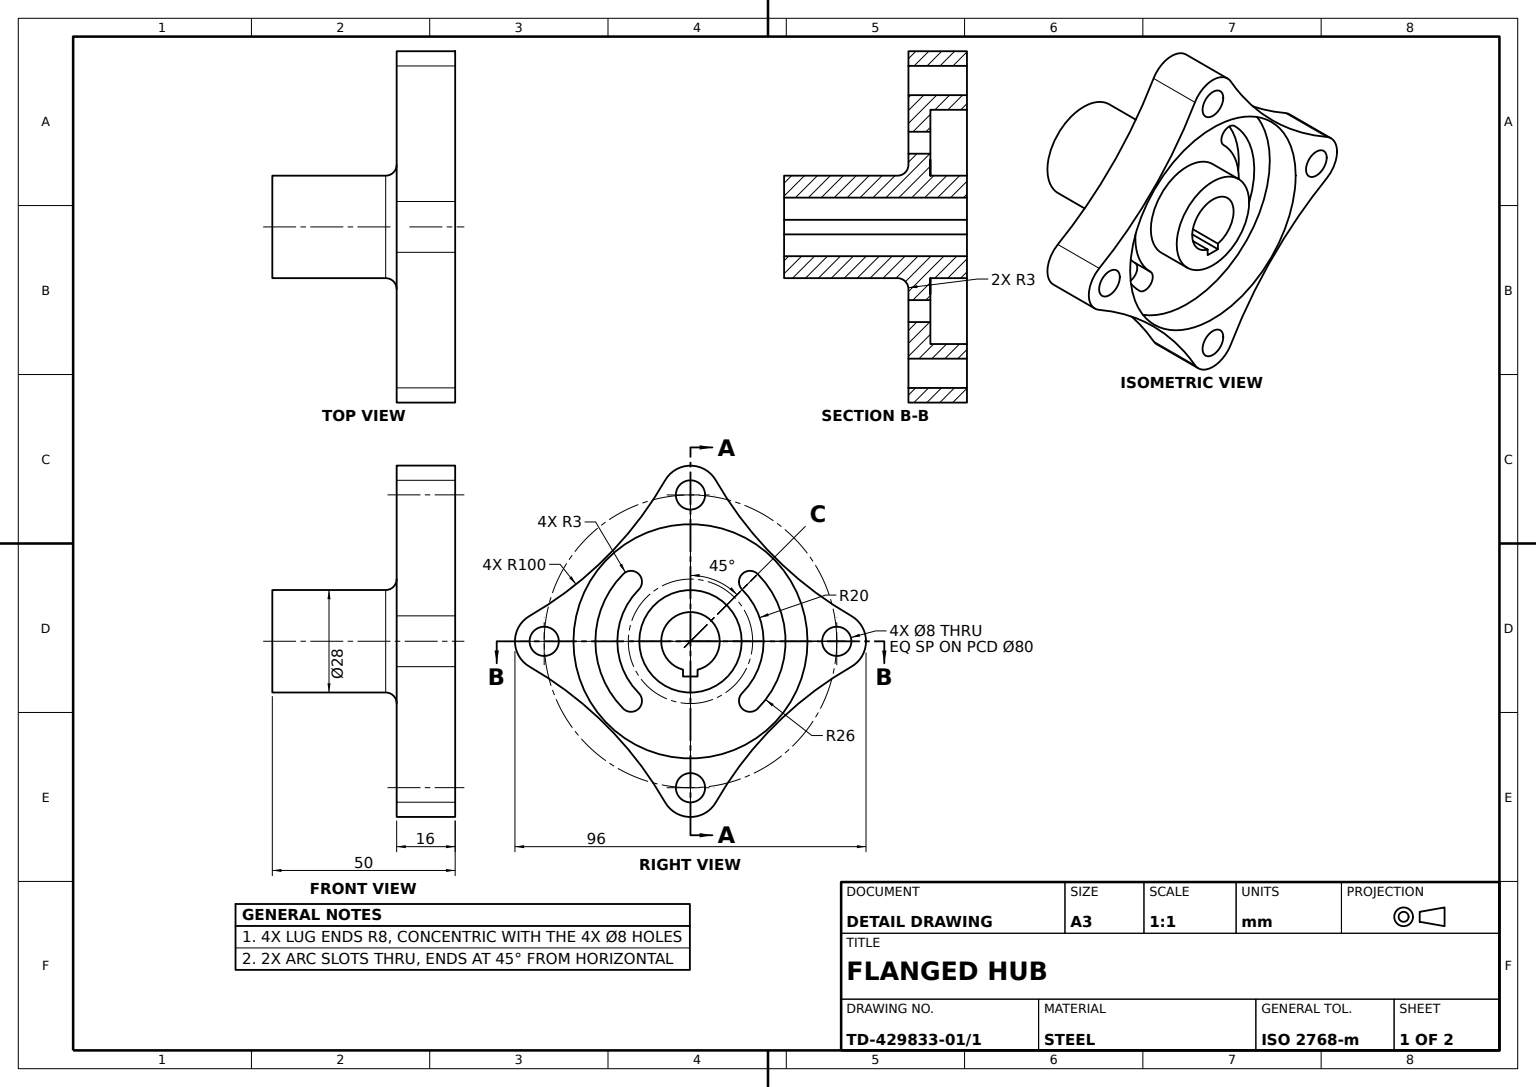
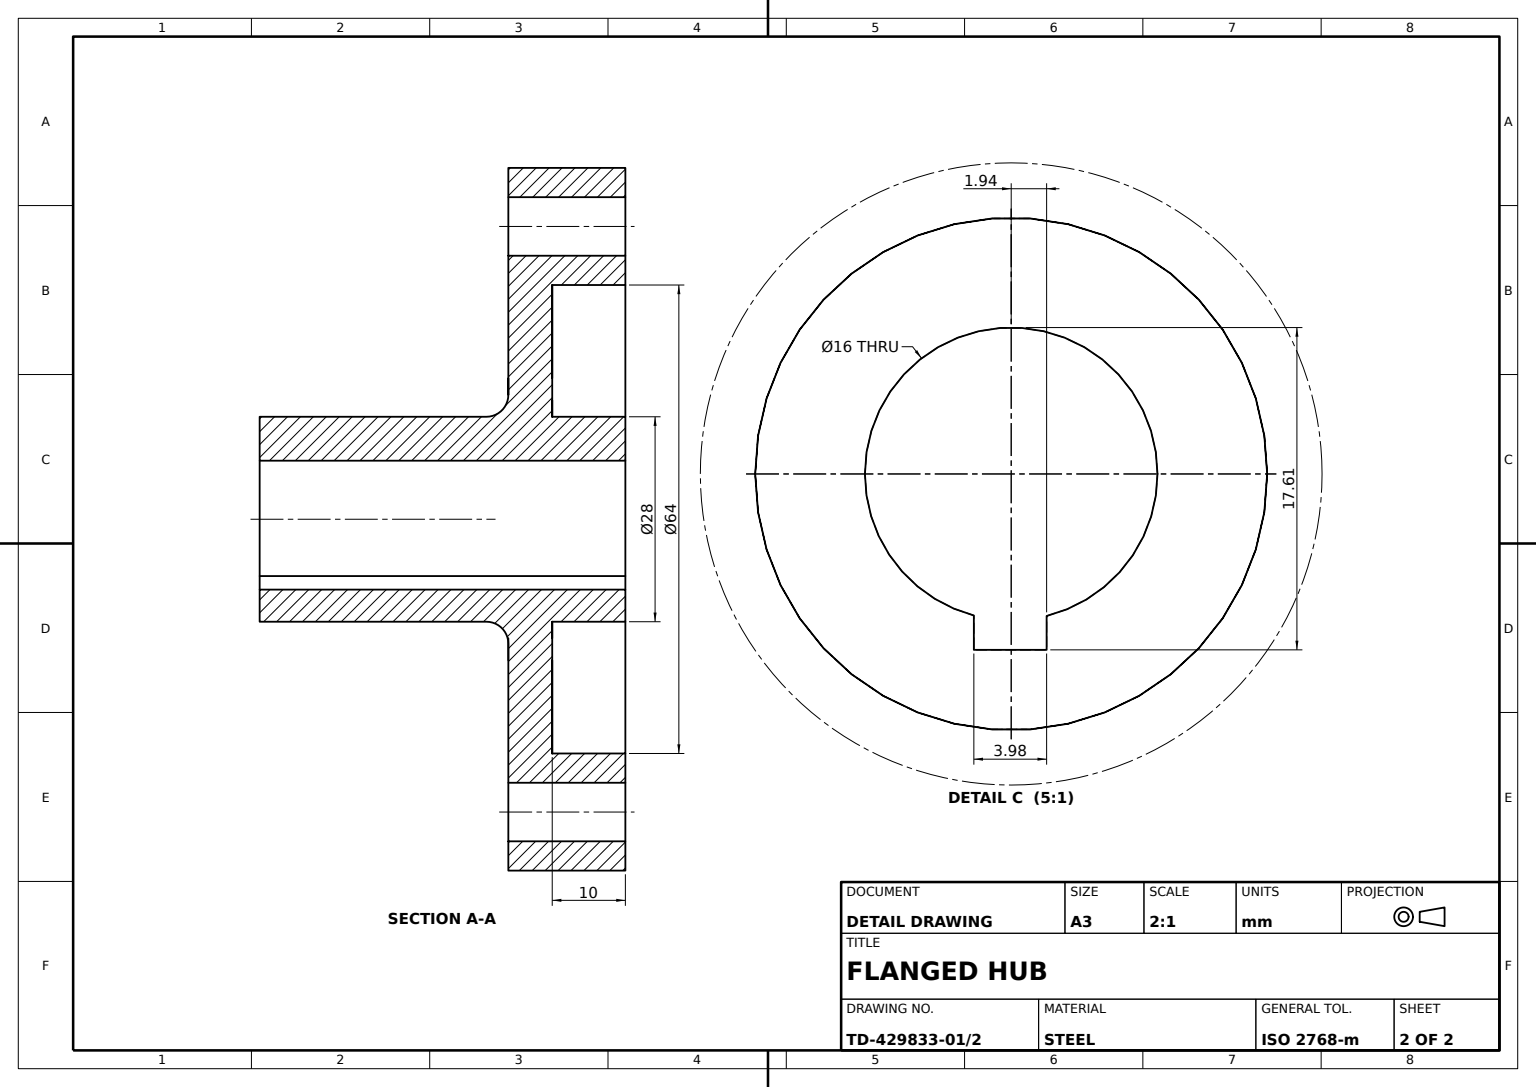
SolidWorks part; units mm, degrees
material "Plain Carbon Steel"
ref_plane "Front Plane" through (0, 0, 0) normal (0, 0, 1) x (1, 0, 0)
ref_plane "Top Plane" through (0, 0, 0) normal (0, 1, 0) x (1, 0, 0)
ref_plane "Right Plane" through (0, 0, 0) normal (1, 0, 0) x (0, 0, -1)
sketch "Flange Profile Sketch" plane through (0, 0, 0) normal (0, 1, 0) x (1, 0, 0)
  line L0 (0, 0) -> (0, 20.431) construction
  line L1 (0, 0) -> (11.6852, 0) construction
  circle A0 centre (0, 0) radius 40 construction
  arc A2 (43.9779, -6.9409) -> (43.9779, 6.9409) centre (40, 0) ccw
  arc A3 (6.9409, 43.9779) -> (-6.9409, 43.9779) centre (0, 40) ccw
  arc A4 (6.9409, 43.9779) -> (43.9779, 6.9409) centre (93.7021, 93.7021) ccw
  arc A5 (-6.9409, 43.9779) -> (-43.9779, 6.9409) centre (-93.7021, 93.7021) cw
  arc A6 (-43.9779, -6.9409) -> (-43.9779, 6.9409) centre (-40, 0) cw
  arc A7 (-6.9409, -43.9779) -> (-43.9779, -6.9409) centre (-93.7021, -93.7021) ccw
  arc A8 (6.9409, -43.9779) -> (-6.9409, -43.9779) centre (0, -40) cw
  arc A9 (6.9409, -43.9779) -> (43.9779, -6.9409) centre (93.7021, -93.7021) cw
  circle A10 centre (40, 0) radius 4
  circle A11 centre (0, -40) radius 4
  circle A12 centre (-40, 0) radius 4
  circle A13 centre (0, 40) radius 4
  dimension "D1" = 80
  dimension "D2" = 8
  dimension "D3" = 16
  dimension "D4" = 100
  dimension "D5" = 4
extrude "Square Flange 100x16" add sketch "Flange Profile Sketch" along normal blind 16
sketch "Recess Sketch Ø64" plane through (0, 16, 0) normal (0, 1, 0) x (1, 0, 0)
  circle A0 centre (0, 0) radius 32
  dimension "D1" = 64
extrude "Recess Ø64x10" cut sketch "Recess Sketch Ø64" against normal blind 10
sketch "Hub Sketch Ø28" plane through (0, 6, 0) normal (0, 1, 0) x (1, 0, 0)
  circle A0 centre (0, 0) radius 14
  dimension "D1" = 28
extrude "Hub Boss Ø28" add sketch "Hub Sketch Ø28" along normal up to surface and the other way blind 40 up to face at (0, 16, 32)
fillet "Hub Fillet R3" radius 3 1 edges at (0, 0, 14)
sketch "Keyed Bore Sketch" plane through (0, 16, 0) normal (0, 1, 0) x (1, 0, 0)
  line L1 (9.6118, 0) -> (9.6118, 1.9375)
  line L2 (9.6118, 1.9375) -> (7.7618, 1.9375)
  line L3 (9.6118, 0) -> (9.6118, -2.0425)
  line L4 (9.6118, -2.0425) -> (7.7349, -2.0425)
  arc A0 (7.7618, 1.9375) -> (7.7349, -2.0425) centre (0, 0) ccw
  dimension "D1" = 8
  dimension "D2" = 3.98
  dimension "D3" = 1.85
  dimension "D4" = 1.9375
extrude "Keyed Bore" cut sketch "Keyed Bore Sketch" against normal through all
sketch "Arc Slots Sketch" plane through (0, 6, 0) normal (0, 1, 0) x (1, 0, 0)
  line L0 (0, 0) -> (0, 32.9222) construction
  line L1 (0, 0) -> (-50.5485, 0) construction
  line L2 (0, 0) -> (-30.8139, 30.8139) construction
  arc A0 (-16.2635, 16.2635) -> (16.2635, 16.2635) centre (0, 0) cw construction
  arc A1 (18.3848, 18.3848) -> (-18.3848, 18.3848) centre (0, 0) ccw
  arc A2 (14.1421, 14.1421) -> (-14.1421, 14.1421) centre (0, 0) ccw
  arc A3 (14.1421, 14.1421) -> (18.3848, 18.3848) centre (16.2635, 16.2635) ccw
  arc A4 (-18.3848, 18.3848) -> (-14.1421, 14.1421) centre (-16.2635, 16.2635) ccw
  arc A5 (-16.2635, -16.2635) -> (16.2635, -16.2635) centre (0, 0) ccw construction
  arc A6 (18.3848, -18.3848) -> (-18.3848, -18.3848) centre (0, 0) cw
  arc A7 (14.1421, -14.1421) -> (-14.1421, -14.1421) centre (0, 0) cw
  arc A8 (14.1421, -14.1421) -> (18.3848, -18.3848) centre (16.2635, -16.2635) cw
  arc A9 (-18.3848, -18.3848) -> (-14.1421, -14.1421) centre (-16.2635, -16.2635) cw
  point P4 (0, 23)
  point P17 (0, -23)
  dimension "D1" = 26
  dimension "D2" = 20
  dimension "D3" = 45
extrude "Arc Slots" cut sketch "Arc Slots Sketch" against normal up to next
